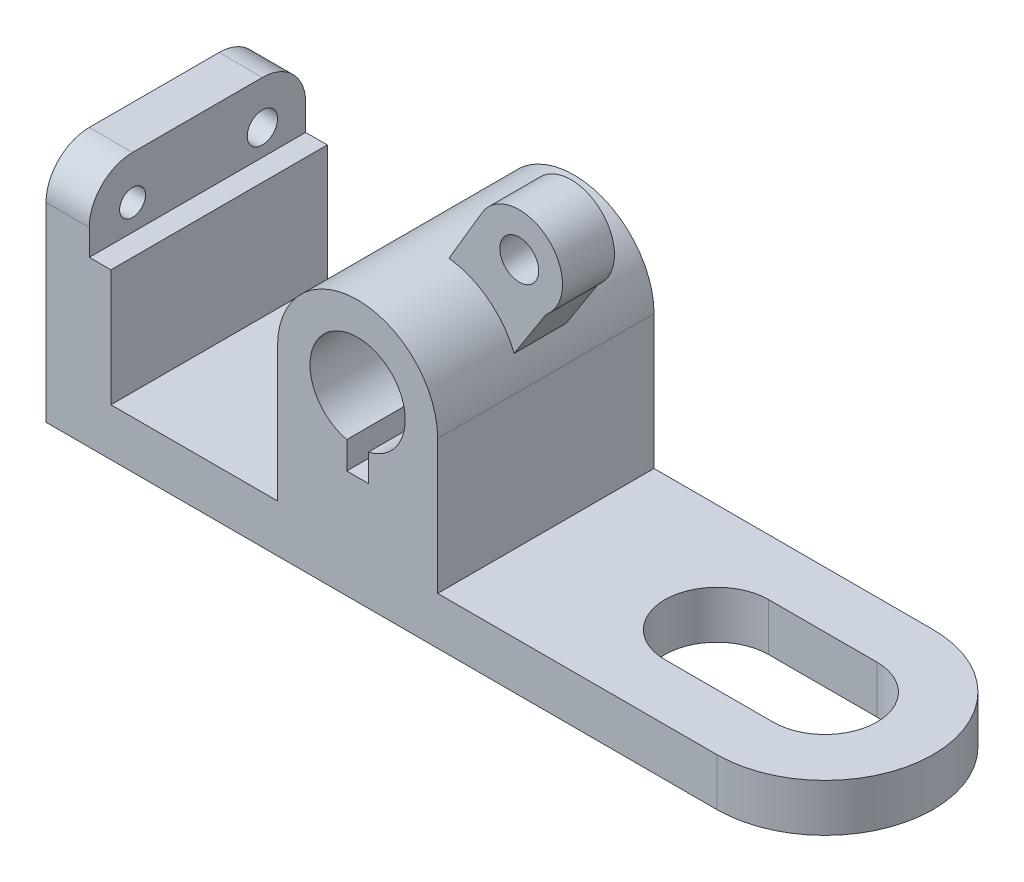
ISO-10303-21;
HEADER;
FILE_DESCRIPTION(('STEP AP214'),'2;1');
FILE_NAME('part.step','',(''),(''),'','','');
FILE_SCHEMA(('AUTOMOTIVE_DESIGN { 1 0 10303 214 1 1 1 1 }'));
ENDSEC;
DATA;
#1=APPLICATION_CONTEXT('core data for automotive mechanical design processes');
#2=APPLICATION_PROTOCOL_DEFINITION('international standard','automotive_design',2000,#1);
#3=PRODUCT_CONTEXT('',#1,'mechanical');
#4=PRODUCT('Part','Part','',(#3));
#5=PRODUCT_RELATED_PRODUCT_CATEGORY('part','',(#4));
#6=PRODUCT_DEFINITION_FORMATION('','',#4);
#7=PRODUCT_DEFINITION_CONTEXT('part definition',#1,'design');
#8=PRODUCT_DEFINITION('design','',#6,#7);
#9=PRODUCT_DEFINITION_SHAPE('','',#8);
#10=(LENGTH_UNIT() NAMED_UNIT(*) SI_UNIT(.MILLI.,.METRE.));
#11=(NAMED_UNIT(*) PLANE_ANGLE_UNIT() SI_UNIT($,.RADIAN.));
#12=(NAMED_UNIT(*) SI_UNIT($,.STERADIAN.) SOLID_ANGLE_UNIT());
#13=UNCERTAINTY_MEASURE_WITH_UNIT(LENGTH_MEASURE(1.E-05),#10,'distance_accuracy_value','');
#14=(GEOMETRIC_REPRESENTATION_CONTEXT(3) GLOBAL_UNCERTAINTY_ASSIGNED_CONTEXT((#13)) GLOBAL_UNIT_ASSIGNED_CONTEXT((#10,
#11,#12)) REPRESENTATION_CONTEXT('',''));
#15=CARTESIAN_POINT('',(0.,0.,0.));
#16=DIRECTION('',(0.,0.,1.));
#17=DIRECTION('',(1.,0.,0.));
#18=AXIS2_PLACEMENT_3D('',#15,#16,#17);
#19=CARTESIAN_POINT('',(-77.5,44.,-15.));
#20=DIRECTION('',(-1.,0.,0.));
#21=DIRECTION('',(0.,0.,1.));
#22=AXIS2_PLACEMENT_3D('',#19,#20,#21);
#23=CYLINDRICAL_SURFACE('',#22,10.);
#24=DIRECTION('',(1.,0.,0.));
#25=VECTOR('',#24,1.);
#26=CARTESIAN_POINT('',(-77.5,44.,-25.));
#27=LINE('',#26,#25);
#28=CARTESIAN_POINT('',(-77.5,44.,-25.));
#29=VERTEX_POINT('',#28);
#30=CARTESIAN_POINT('',(-67.5,44.,-25.));
#31=VERTEX_POINT('',#30);
#32=EDGE_CURVE('E419',#29,#31,#27,.T.);
#33=ORIENTED_EDGE('',*,*,#32,.F.);
#34=CARTESIAN_POINT('',(-77.5,44.,-15.));
#35=DIRECTION('',(1.,0.,0.));
#36=DIRECTION('',(0.,0.,-1.));
#37=AXIS2_PLACEMENT_3D('',#34,#35,#36);
#38=CIRCLE('',#37,10.);
#39=CARTESIAN_POINT('',(-77.5,54.,-15.));
#40=VERTEX_POINT('',#39);
#41=EDGE_CURVE('E11',#40,#29,#38,.F.);
#42=ORIENTED_EDGE('',*,*,#41,.F.);
#43=DIRECTION('',(1.,0.,0.));
#44=VECTOR('',#43,1.);
#45=CARTESIAN_POINT('',(-77.5,54.,-15.));
#46=LINE('',#45,#44);
#47=CARTESIAN_POINT('',(-67.5,54.,-15.));
#48=VERTEX_POINT('',#47);
#49=EDGE_CURVE('E47',#48,#40,#46,.F.);
#50=ORIENTED_EDGE('',*,*,#49,.F.);
#51=CARTESIAN_POINT('',(-67.5,44.,-15.));
#52=DIRECTION('',(1.,0.,0.));
#53=DIRECTION('',(0.,0.,-1.));
#54=AXIS2_PLACEMENT_3D('',#51,#52,#53);
#55=CIRCLE('',#54,10.);
#56=EDGE_CURVE('E421',#31,#48,#55,.T.);
#57=ORIENTED_EDGE('',*,*,#56,.F.);
#58=EDGE_LOOP('',(#33,#42,#50,#57));
#59=FACE_BOUND('',#58,.T.);
#60=ADVANCED_FACE('F41',(#59),#23,.T.);
#61=CARTESIAN_POINT('',(77.5,44.,15.));
#62=DIRECTION('',(1.,0.,0.));
#63=DIRECTION('',(0.,0.,-1.));
#64=AXIS2_PLACEMENT_3D('',#61,#62,#63);
#65=CYLINDRICAL_SURFACE('',#64,10.);
#66=DIRECTION('',(-1.,0.,0.));
#67=VECTOR('',#66,1.);
#68=CARTESIAN_POINT('',(77.5,44.,25.));
#69=LINE('',#68,#67);
#70=CARTESIAN_POINT('',(-67.5,44.,25.));
#71=VERTEX_POINT('',#70);
#72=CARTESIAN_POINT('',(-77.5,44.,25.));
#73=VERTEX_POINT('',#72);
#74=EDGE_CURVE('E413',#71,#73,#69,.T.);
#75=ORIENTED_EDGE('',*,*,#74,.F.);
#76=CARTESIAN_POINT('',(-67.5,44.,15.));
#77=DIRECTION('',(1.,0.,0.));
#78=DIRECTION('',(0.,0.,-1.));
#79=AXIS2_PLACEMENT_3D('',#76,#77,#78);
#80=CIRCLE('',#79,10.);
#81=CARTESIAN_POINT('',(-67.5,54.,15.));
#82=VERTEX_POINT('',#81);
#83=EDGE_CURVE('E240',#82,#71,#80,.T.);
#84=ORIENTED_EDGE('',*,*,#83,.F.);
#85=DIRECTION('',(-1.,0.,0.));
#86=VECTOR('',#85,1.);
#87=CARTESIAN_POINT('',(77.5,54.,15.));
#88=LINE('',#87,#86);
#89=CARTESIAN_POINT('',(-77.5,54.,15.));
#90=VERTEX_POINT('',#89);
#91=EDGE_CURVE('E412',#90,#82,#88,.F.);
#92=ORIENTED_EDGE('',*,*,#91,.F.);
#93=CARTESIAN_POINT('',(-77.5,44.,15.));
#94=DIRECTION('',(1.,0.,0.));
#95=DIRECTION('',(0.,0.,-1.));
#96=AXIS2_PLACEMENT_3D('',#93,#94,#95);
#97=CIRCLE('',#96,10.);
#98=EDGE_CURVE('E420',#73,#90,#97,.F.);
#99=ORIENTED_EDGE('',*,*,#98,.F.);
#100=EDGE_LOOP('',(#75,#84,#92,#99));
#101=FACE_BOUND('',#100,.T.);
#102=ADVANCED_FACE('F451',(#101),#65,.T.);
#103=CARTESIAN_POINT('',(77.5,11.,0.));
#104=DIRECTION('',(0.,1.,0.));
#105=DIRECTION('',(0.,0.,1.));
#106=AXIS2_PLACEMENT_3D('',#103,#104,#105);
#107=PLANE('',#106);
#108=DIRECTION('',(-1.,0.,0.));
#109=VECTOR('',#108,1.);
#110=CARTESIAN_POINT('',(-77.5,11.,-25.));
#111=LINE('',#110,#109);
#112=CARTESIAN_POINT('',(-24.,11.,-25.));
#113=VERTEX_POINT('',#112);
#114=CARTESIAN_POINT('',(-62.5,11.,-25.));
#115=VERTEX_POINT('',#114);
#116=EDGE_CURVE('E368',#113,#115,#111,.T.);
#117=ORIENTED_EDGE('',*,*,#116,.T.);
#118=DIRECTION('',(0.,0.,-1.));
#119=VECTOR('',#118,1.);
#120=CARTESIAN_POINT('',(-62.5,11.,25.));
#121=LINE('',#120,#119);
#122=CARTESIAN_POINT('',(-62.5,11.,25.));
#123=VERTEX_POINT('',#122);
#124=EDGE_CURVE('E225',#123,#115,#121,.T.);
#125=ORIENTED_EDGE('',*,*,#124,.F.);
#126=DIRECTION('',(1.,0.,0.));
#127=VECTOR('',#126,1.);
#128=CARTESIAN_POINT('',(77.5,11.,25.));
#129=LINE('',#128,#127);
#130=CARTESIAN_POINT('',(-24.,11.,25.));
#131=VERTEX_POINT('',#130);
#132=EDGE_CURVE('E367',#123,#131,#129,.T.);
#133=ORIENTED_EDGE('',*,*,#132,.T.);
#134=DIRECTION('',(0.,0.,1.));
#135=VECTOR('',#134,1.);
#136=CARTESIAN_POINT('',(-24.,11.,-25.));
#137=LINE('',#136,#135);
#138=EDGE_CURVE('E356',#113,#131,#137,.T.);
#139=ORIENTED_EDGE('',*,*,#138,.F.);
#140=EDGE_LOOP('',(#117,#125,#133,#139));
#141=FACE_BOUND('',#140,.T.);
#142=ADVANCED_FACE('F494',(#141),#107,.T.);
#143=CARTESIAN_POINT('',(77.5,11.,0.));
#144=DIRECTION('',(0.,1.,0.));
#145=DIRECTION('',(0.,0.,1.));
#146=AXIS2_PLACEMENT_3D('',#143,#144,#145);
#147=CIRCLE('',#146,12.);
#148=CARTESIAN_POINT('',(77.5000000000001,11.,12.));
#149=VERTEX_POINT('',#148);
#150=CARTESIAN_POINT('',(77.5,11.,-12.));
#151=VERTEX_POINT('',#150);
#152=EDGE_CURVE('E259',#149,#151,#147,.T.);
#153=ORIENTED_EDGE('',*,*,#152,.F.);
#154=DIRECTION('',(1.,0.,0.));
#155=VECTOR('',#154,1.);
#156=CARTESIAN_POINT('',(52.5,11.,12.));
#157=LINE('',#156,#155);
#158=CARTESIAN_POINT('',(52.5,11.,12.));
#159=VERTEX_POINT('',#158);
#160=EDGE_CURVE('E265',#159,#149,#157,.T.);
#161=ORIENTED_EDGE('',*,*,#160,.F.);
#162=CARTESIAN_POINT('',(52.5,11.,0.));
#163=DIRECTION('',(0.,1.,0.));
#164=DIRECTION('',(0.,0.,1.));
#165=AXIS2_PLACEMENT_3D('',#162,#163,#164);
#166=CIRCLE('',#165,12.);
#167=CARTESIAN_POINT('',(52.5,11.,-12.));
#168=VERTEX_POINT('',#167);
#169=EDGE_CURVE('E263',#168,#159,#166,.T.);
#170=ORIENTED_EDGE('',*,*,#169,.F.);
#171=DIRECTION('',(-1.,0.,0.));
#172=VECTOR('',#171,1.);
#173=CARTESIAN_POINT('',(52.5,11.,-12.));
#174=LINE('',#173,#172);
#175=EDGE_CURVE('E260',#151,#168,#174,.T.);
#176=ORIENTED_EDGE('',*,*,#175,.F.);
#177=EDGE_LOOP('',(#153,#161,#170,#176));
#178=FACE_BOUND('',#177,.T.);
#179=CARTESIAN_POINT('',(77.5,11.,-25.));
#180=VERTEX_POINT('',#179);
#181=CARTESIAN_POINT('',(13.,11.,-25.));
#182=VERTEX_POINT('',#181);
#183=EDGE_CURVE('E364',#180,#182,#111,.T.);
#184=ORIENTED_EDGE('',*,*,#183,.T.);
#185=DIRECTION('',(0.,0.,1.));
#186=VECTOR('',#185,1.);
#187=CARTESIAN_POINT('',(13.,11.,-25.));
#188=LINE('',#187,#186);
#189=CARTESIAN_POINT('',(13.,11.,25.));
#190=VERTEX_POINT('',#189);
#191=EDGE_CURVE('E352',#182,#190,#188,.T.);
#192=ORIENTED_EDGE('',*,*,#191,.T.);
#193=CARTESIAN_POINT('',(77.5,11.,25.));
#194=VERTEX_POINT('',#193);
#195=EDGE_CURVE('E370',#190,#194,#129,.T.);
#196=ORIENTED_EDGE('',*,*,#195,.T.);
#197=CARTESIAN_POINT('',(77.5,11.,0.));
#198=DIRECTION('',(0.,1.,0.));
#199=DIRECTION('',(0.,0.,1.));
#200=AXIS2_PLACEMENT_3D('',#197,#198,#199);
#201=CIRCLE('',#200,25.);
#202=EDGE_CURVE('E371',#194,#180,#201,.T.);
#203=ORIENTED_EDGE('',*,*,#202,.T.);
#204=EDGE_LOOP('',(#184,#192,#196,#203));
#205=FACE_BOUND('',#204,.T.);
#206=ADVANCED_FACE('F466',(#178,#205),#107,.T.);
#207=CARTESIAN_POINT('',(-77.5,11.,-25.));
#208=DIRECTION('',(0.,0.,1.));
#209=DIRECTION('',(1.,0.,0.));
#210=AXIS2_PLACEMENT_3D('',#207,#208,#209);
#211=PLANE('',#210);
#212=DIRECTION('',(-1.,0.,0.));
#213=VECTOR('',#212,1.);
#214=CARTESIAN_POINT('',(-5.5,25.,-25.));
#215=LINE('',#214,#213);
#216=CARTESIAN_POINT('',(-3.,25.,-25.));
#217=VERTEX_POINT('',#216);
#218=CARTESIAN_POINT('',(-8.,25.,-25.));
#219=VERTEX_POINT('',#218);
#220=EDGE_CURVE('E319',#217,#219,#215,.T.);
#221=ORIENTED_EDGE('',*,*,#220,.F.);
#222=DIRECTION('',(0.,1.,0.));
#223=VECTOR('',#222,1.);
#224=CARTESIAN_POINT('',(-3.,25.,-25.));
#225=LINE('',#224,#223);
#226=CARTESIAN_POINT('',(-3.,31.2878573571857,-25.));
#227=VERTEX_POINT('',#226);
#228=EDGE_CURVE('E308',#217,#227,#225,.T.);
#229=ORIENTED_EDGE('',*,*,#228,.T.);
#230=CARTESIAN_POINT('',(-5.50000000000001,42.,-25.));
#231=DIRECTION('',(0.,0.,1.));
#232=DIRECTION('',(1.,0.,0.));
#233=AXIS2_PLACEMENT_3D('',#230,#231,#232);
#234=CIRCLE('',#233,11.);
#235=CARTESIAN_POINT('',(-8.,31.2878573571857,-25.));
#236=VERTEX_POINT('',#235);
#237=EDGE_CURVE('E311',#227,#236,#234,.T.);
#238=ORIENTED_EDGE('',*,*,#237,.T.);
#239=DIRECTION('',(0.,1.,0.));
#240=VECTOR('',#239,1.);
#241=CARTESIAN_POINT('',(-8.,25.,-25.));
#242=LINE('',#241,#240);
#243=EDGE_CURVE('E314',#219,#236,#242,.T.);
#244=ORIENTED_EDGE('',*,*,#243,.F.);
#245=EDGE_LOOP('',(#221,#229,#238,#244));
#246=FACE_BOUND('',#245,.T.);
#247=DIRECTION('',(0.,-1.,0.));
#248=VECTOR('',#247,1.);
#249=CARTESIAN_POINT('',(-77.5,11.,-25.));
#250=LINE('',#249,#248);
#251=CARTESIAN_POINT('',(-77.5,0.,-25.));
#252=VERTEX_POINT('',#251);
#253=EDGE_CURVE('E387',#29,#252,#250,.T.);
#254=ORIENTED_EDGE('',*,*,#253,.F.);
#255=ORIENTED_EDGE('',*,*,#32,.T.);
#256=DIRECTION('',(0.,1.,0.));
#257=VECTOR('',#256,1.);
#258=CARTESIAN_POINT('',(-67.5,38.,-25.));
#259=LINE('',#258,#257);
#260=CARTESIAN_POINT('',(-67.5,38.,-25.));
#261=VERTEX_POINT('',#260);
#262=EDGE_CURVE('E231',#261,#31,#259,.T.);
#263=ORIENTED_EDGE('',*,*,#262,.F.);
#264=DIRECTION('',(-1.,0.,0.));
#265=VECTOR('',#264,1.);
#266=CARTESIAN_POINT('',(-62.5,38.,-25.));
#267=LINE('',#266,#265);
#268=CARTESIAN_POINT('',(-62.5,38.,-25.));
#269=VERTEX_POINT('',#268);
#270=EDGE_CURVE('E226',#269,#261,#267,.T.);
#271=ORIENTED_EDGE('',*,*,#270,.F.);
#272=DIRECTION('',(0.,-1.,0.));
#273=VECTOR('',#272,1.);
#274=CARTESIAN_POINT('',(-62.5,38.,-25.));
#275=LINE('',#274,#273);
#276=EDGE_CURVE('E249',#269,#115,#275,.T.);
#277=ORIENTED_EDGE('',*,*,#276,.T.);
#278=ORIENTED_EDGE('',*,*,#116,.F.);
#279=DIRECTION('',(0.,-1.,0.));
#280=VECTOR('',#279,1.);
#281=CARTESIAN_POINT('',(-24.,0.,-25.));
#282=LINE('',#281,#280);
#283=CARTESIAN_POINT('',(-24.,42.,-25.));
#284=VERTEX_POINT('',#283);
#285=EDGE_CURVE('E342',#284,#113,#282,.T.);
#286=ORIENTED_EDGE('',*,*,#285,.F.);
#287=CARTESIAN_POINT('',(-5.50000000000001,42.,-25.));
#288=DIRECTION('',(0.,0.,1.));
#289=DIRECTION('',(1.,0.,0.));
#290=AXIS2_PLACEMENT_3D('',#287,#288,#289);
#291=CIRCLE('',#290,18.5);
#292=CARTESIAN_POINT('',(13.,42.,-25.));
#293=VERTEX_POINT('',#292);
#294=EDGE_CURVE('E344',#293,#284,#291,.T.);
#295=ORIENTED_EDGE('',*,*,#294,.F.);
#296=DIRECTION('',(0.,-1.,0.));
#297=VECTOR('',#296,1.);
#298=CARTESIAN_POINT('',(13.,0.,-25.));
#299=LINE('',#298,#297);
#300=EDGE_CURVE('E339',#293,#182,#299,.T.);
#301=ORIENTED_EDGE('',*,*,#300,.T.);
#302=ORIENTED_EDGE('',*,*,#183,.F.);
#303=DIRECTION('',(0.,-1.,0.));
#304=VECTOR('',#303,1.);
#305=CARTESIAN_POINT('',(77.5,11.,-25.));
#306=LINE('',#305,#304);
#307=CARTESIAN_POINT('',(77.5,0.,-25.));
#308=VERTEX_POINT('',#307);
#309=EDGE_CURVE('E373',#180,#308,#306,.T.);
#310=ORIENTED_EDGE('',*,*,#309,.T.);
#311=DIRECTION('',(-1.,0.,0.));
#312=VECTOR('',#311,1.);
#313=CARTESIAN_POINT('',(-77.5,0.,-25.));
#314=LINE('',#313,#312);
#315=EDGE_CURVE('E357',#308,#252,#314,.T.);
#316=ORIENTED_EDGE('',*,*,#315,.T.);
#317=EDGE_LOOP('',(#254,#255,#263,#271,#277,#278,#286,#295,#301,#302,#310,#316));
#318=FACE_BOUND('',#317,.T.);
#319=ADVANCED_FACE('F445',(#246,#318),#211,.F.);
#320=CARTESIAN_POINT('',(-77.5,11.,-25.));
#321=DIRECTION('',(1.,0.,0.));
#322=DIRECTION('',(0.,0.,-1.));
#323=AXIS2_PLACEMENT_3D('',#320,#321,#322);
#324=PLANE('',#323);
#325=CARTESIAN_POINT('',(-77.5,44.,-15.));
#326=DIRECTION('',(-1.,0.,0.));
#327=DIRECTION('',(0.,0.,1.));
#328=AXIS2_PLACEMENT_3D('',#325,#326,#327);
#329=CIRCLE('',#328,3.5);
#330=CARTESIAN_POINT('',(-77.5,44.,-11.5));
#331=VERTEX_POINT('',#330);
#332=EDGE_CURVE('E428',#331,#331,#329,.T.);
#333=ORIENTED_EDGE('',*,*,#332,.F.);
#334=EDGE_LOOP('',(#333));
#335=FACE_BOUND('',#334,.T.);
#336=CARTESIAN_POINT('',(-77.5,44.,15.));
#337=DIRECTION('',(-1.,0.,0.));
#338=DIRECTION('',(0.,0.,1.));
#339=AXIS2_PLACEMENT_3D('',#336,#337,#338);
#340=CIRCLE('',#339,3.);
#341=CARTESIAN_POINT('',(-77.5,44.,18.));
#342=VERTEX_POINT('',#341);
#343=EDGE_CURVE('E427',#342,#342,#340,.T.);
#344=ORIENTED_EDGE('',*,*,#343,.F.);
#345=EDGE_LOOP('',(#344));
#346=FACE_BOUND('',#345,.T.);
#347=DIRECTION('',(0.,0.,1.));
#348=VECTOR('',#347,1.);
#349=CARTESIAN_POINT('',(-77.5,54.,-25.));
#350=LINE('',#349,#348);
#351=EDGE_CURVE('E244',#40,#90,#350,.T.);
#352=ORIENTED_EDGE('',*,*,#351,.F.);
#353=ORIENTED_EDGE('',*,*,#41,.T.);
#354=ORIENTED_EDGE('',*,*,#253,.T.);
#355=DIRECTION('',(0.,0.,1.));
#356=VECTOR('',#355,1.);
#357=CARTESIAN_POINT('',(-77.5,0.,-25.));
#358=LINE('',#357,#356);
#359=CARTESIAN_POINT('',(-77.5,0.,25.));
#360=VERTEX_POINT('',#359);
#361=EDGE_CURVE('E376',#252,#360,#358,.T.);
#362=ORIENTED_EDGE('',*,*,#361,.T.);
#363=DIRECTION('',(0.,-1.,0.));
#364=VECTOR('',#363,1.);
#365=CARTESIAN_POINT('',(-77.5,11.,25.));
#366=LINE('',#365,#364);
#367=EDGE_CURVE('E390',#73,#360,#366,.T.);
#368=ORIENTED_EDGE('',*,*,#367,.F.);
#369=ORIENTED_EDGE('',*,*,#98,.T.);
#370=EDGE_LOOP('',(#352,#353,#354,#362,#368,#369));
#371=FACE_BOUND('',#370,.T.);
#372=ADVANCED_FACE('F437',(#335,#346,#371),#324,.F.);
#373=CARTESIAN_POINT('',(77.5,11.,25.));
#374=DIRECTION('',(0.,0.,-1.));
#375=DIRECTION('',(-1.,0.,0.));
#376=AXIS2_PLACEMENT_3D('',#373,#374,#375);
#377=PLANE('',#376);
#378=CARTESIAN_POINT('',(-5.50000000000001,42.,25.));
#379=DIRECTION('',(0.,0.,1.));
#380=DIRECTION('',(1.,0.,0.));
#381=AXIS2_PLACEMENT_3D('',#378,#379,#380);
#382=CIRCLE('',#381,11.);
#383=CARTESIAN_POINT('',(-3.,31.2878573571857,25.));
#384=VERTEX_POINT('',#383);
#385=CARTESIAN_POINT('',(-8.,31.2878573571857,25.));
#386=VERTEX_POINT('',#385);
#387=EDGE_CURVE('E321',#384,#386,#382,.T.);
#388=ORIENTED_EDGE('',*,*,#387,.F.);
#389=DIRECTION('',(0.,1.,0.));
#390=VECTOR('',#389,1.);
#391=CARTESIAN_POINT('',(-3.,25.,25.));
#392=LINE('',#391,#390);
#393=CARTESIAN_POINT('',(-3.,25.,25.));
#394=VERTEX_POINT('',#393);
#395=EDGE_CURVE('E310',#394,#384,#392,.T.);
#396=ORIENTED_EDGE('',*,*,#395,.F.);
#397=DIRECTION('',(1.,0.,0.));
#398=VECTOR('',#397,1.);
#399=CARTESIAN_POINT('',(-5.5,25.,25.));
#400=LINE('',#399,#398);
#401=CARTESIAN_POINT('',(-8.,25.,25.));
#402=VERTEX_POINT('',#401);
#403=EDGE_CURVE('E315',#402,#394,#400,.T.);
#404=ORIENTED_EDGE('',*,*,#403,.F.);
#405=DIRECTION('',(0.,1.,0.));
#406=VECTOR('',#405,1.);
#407=CARTESIAN_POINT('',(-8.,25.,25.));
#408=LINE('',#407,#406);
#409=EDGE_CURVE('E322',#402,#386,#408,.T.);
#410=ORIENTED_EDGE('',*,*,#409,.T.);
#411=EDGE_LOOP('',(#388,#396,#404,#410));
#412=FACE_BOUND('',#411,.T.);
#413=DIRECTION('',(0.,1.,0.));
#414=VECTOR('',#413,1.);
#415=CARTESIAN_POINT('',(-67.5,38.,25.));
#416=LINE('',#415,#414);
#417=CARTESIAN_POINT('',(-67.5,38.,25.));
#418=VERTEX_POINT('',#417);
#419=EDGE_CURVE('E212',#418,#71,#416,.T.);
#420=ORIENTED_EDGE('',*,*,#419,.T.);
#421=ORIENTED_EDGE('',*,*,#74,.T.);
#422=ORIENTED_EDGE('',*,*,#367,.T.);
#423=DIRECTION('',(1.,0.,0.));
#424=VECTOR('',#423,1.);
#425=CARTESIAN_POINT('',(77.5,0.,25.));
#426=LINE('',#425,#424);
#427=CARTESIAN_POINT('',(77.5,0.,25.));
#428=VERTEX_POINT('',#427);
#429=EDGE_CURVE('E378',#360,#428,#426,.T.);
#430=ORIENTED_EDGE('',*,*,#429,.T.);
#431=DIRECTION('',(0.,-1.,0.));
#432=VECTOR('',#431,1.);
#433=CARTESIAN_POINT('',(77.5,11.,25.));
#434=LINE('',#433,#432);
#435=EDGE_CURVE('E383',#194,#428,#434,.T.);
#436=ORIENTED_EDGE('',*,*,#435,.F.);
#437=ORIENTED_EDGE('',*,*,#195,.F.);
#438=DIRECTION('',(0.,-1.,0.));
#439=VECTOR('',#438,1.);
#440=CARTESIAN_POINT('',(13.,0.,25.));
#441=LINE('',#440,#439);
#442=CARTESIAN_POINT('',(13.,42.,25.));
#443=VERTEX_POINT('',#442);
#444=EDGE_CURVE('E335',#443,#190,#441,.T.);
#445=ORIENTED_EDGE('',*,*,#444,.F.);
#446=CARTESIAN_POINT('',(-5.50000000000001,42.,25.));
#447=DIRECTION('',(0.,0.,1.));
#448=DIRECTION('',(1.,0.,0.));
#449=AXIS2_PLACEMENT_3D('',#446,#447,#448);
#450=CIRCLE('',#449,18.5);
#451=CARTESIAN_POINT('',(-24.,42.,25.));
#452=VERTEX_POINT('',#451);
#453=EDGE_CURVE('E350',#443,#452,#450,.T.);
#454=ORIENTED_EDGE('',*,*,#453,.T.);
#455=DIRECTION('',(0.,-1.,0.));
#456=VECTOR('',#455,1.);
#457=CARTESIAN_POINT('',(-24.,0.,25.));
#458=LINE('',#457,#456);
#459=EDGE_CURVE('E341',#452,#131,#458,.T.);
#460=ORIENTED_EDGE('',*,*,#459,.T.);
#461=ORIENTED_EDGE('',*,*,#132,.F.);
#462=DIRECTION('',(0.,-1.,0.));
#463=VECTOR('',#462,1.);
#464=CARTESIAN_POINT('',(-62.5,38.,25.));
#465=LINE('',#464,#463);
#466=CARTESIAN_POINT('',(-62.5,38.,25.));
#467=VERTEX_POINT('',#466);
#468=EDGE_CURVE('E217',#467,#123,#465,.T.);
#469=ORIENTED_EDGE('',*,*,#468,.F.);
#470=DIRECTION('',(1.,0.,0.));
#471=VECTOR('',#470,1.);
#472=CARTESIAN_POINT('',(-77.5,38.,25.));
#473=LINE('',#472,#471);
#474=EDGE_CURVE('E208',#418,#467,#473,.T.);
#475=ORIENTED_EDGE('',*,*,#474,.F.);
#476=EDGE_LOOP('',(#420,#421,#422,#430,#436,#437,#445,#454,#460,#461,#469,#475));
#477=FACE_BOUND('',#476,.T.);
#478=ADVANCED_FACE('F211',(#412,#477),#377,.F.);
#479=CARTESIAN_POINT('',(77.5,11.,0.));
#480=DIRECTION('',(0.,-1.,0.));
#481=DIRECTION('',(0.,0.,-1.));
#482=AXIS2_PLACEMENT_3D('',#479,#480,#481);
#483=CYLINDRICAL_SURFACE('',#482,25.);
#484=CARTESIAN_POINT('',(77.5,0.,0.));
#485=DIRECTION('',(0.,1.,0.));
#486=DIRECTION('',(0.,0.,1.));
#487=AXIS2_PLACEMENT_3D('',#484,#485,#486);
#488=CIRCLE('',#487,25.);
#489=EDGE_CURVE('E382',#428,#308,#488,.T.);
#490=ORIENTED_EDGE('',*,*,#489,.T.);
#491=ORIENTED_EDGE('',*,*,#309,.F.);
#492=ORIENTED_EDGE('',*,*,#202,.F.);
#493=ORIENTED_EDGE('',*,*,#435,.T.);
#494=EDGE_LOOP('',(#490,#491,#492,#493));
#495=FACE_BOUND('',#494,.T.);
#496=ADVANCED_FACE('F462',(#495),#483,.T.);
#497=CARTESIAN_POINT('',(77.5,0.,0.));
#498=DIRECTION('',(0.,1.,0.));
#499=DIRECTION('',(0.,0.,1.));
#500=AXIS2_PLACEMENT_3D('',#497,#498,#499);
#501=PLANE('',#500);
#502=DIRECTION('',(1.,0.,0.));
#503=VECTOR('',#502,1.);
#504=CARTESIAN_POINT('',(77.5,0.,12.));
#505=LINE('',#504,#503);
#506=CARTESIAN_POINT('',(52.5,0.,12.));
#507=VERTEX_POINT('',#506);
#508=CARTESIAN_POINT('',(77.5000000000001,0.,12.));
#509=VERTEX_POINT('',#508);
#510=EDGE_CURVE('E403',#507,#509,#505,.T.);
#511=ORIENTED_EDGE('',*,*,#510,.T.);
#512=CARTESIAN_POINT('',(77.5,0.,0.));
#513=DIRECTION('',(0.,1.,0.));
#514=DIRECTION('',(0.,0.,1.));
#515=AXIS2_PLACEMENT_3D('',#512,#513,#514);
#516=CIRCLE('',#515,12.);
#517=CARTESIAN_POINT('',(77.5,0.,-12.));
#518=VERTEX_POINT('',#517);
#519=EDGE_CURVE('E410',#509,#518,#516,.T.);
#520=ORIENTED_EDGE('',*,*,#519,.T.);
#521=DIRECTION('',(-1.,0.,0.));
#522=VECTOR('',#521,1.);
#523=CARTESIAN_POINT('',(77.5,0.,-12.));
#524=LINE('',#523,#522);
#525=CARTESIAN_POINT('',(52.5,0.,-12.));
#526=VERTEX_POINT('',#525);
#527=EDGE_CURVE('E400',#518,#526,#524,.T.);
#528=ORIENTED_EDGE('',*,*,#527,.T.);
#529=CARTESIAN_POINT('',(52.5,0.,0.));
#530=DIRECTION('',(0.,1.,0.));
#531=DIRECTION('',(0.,0.,1.));
#532=AXIS2_PLACEMENT_3D('',#529,#530,#531);
#533=CIRCLE('',#532,12.);
#534=EDGE_CURVE('E405',#526,#507,#533,.T.);
#535=ORIENTED_EDGE('',*,*,#534,.T.);
#536=EDGE_LOOP('',(#511,#520,#528,#535));
#537=FACE_BOUND('',#536,.T.);
#538=ORIENTED_EDGE('',*,*,#315,.F.);
#539=ORIENTED_EDGE('',*,*,#489,.F.);
#540=ORIENTED_EDGE('',*,*,#429,.F.);
#541=ORIENTED_EDGE('',*,*,#361,.F.);
#542=EDGE_LOOP('',(#538,#539,#540,#541));
#543=FACE_BOUND('',#542,.T.);
#544=ADVANCED_FACE('F460',(#537,#543),#501,.F.);
#545=CARTESIAN_POINT('',(13.,0.,-25.));
#546=DIRECTION('',(-1.,0.,0.));
#547=DIRECTION('',(0.,-1.,0.));
#548=AXIS2_PLACEMENT_3D('',#545,#546,#547);
#549=PLANE('',#548);
#550=ORIENTED_EDGE('',*,*,#444,.T.);
#551=ORIENTED_EDGE('',*,*,#191,.F.);
#552=ORIENTED_EDGE('',*,*,#300,.F.);
#553=DIRECTION('',(0.,0.,1.));
#554=VECTOR('',#553,1.);
#555=CARTESIAN_POINT('',(13.,42.,-25.));
#556=LINE('',#555,#554);
#557=EDGE_CURVE('E349',#293,#443,#556,.T.);
#558=ORIENTED_EDGE('',*,*,#557,.T.);
#559=EDGE_LOOP('',(#550,#551,#552,#558));
#560=FACE_BOUND('',#559,.T.);
#561=ADVANCED_FACE('F507',(#560),#549,.F.);
#562=CARTESIAN_POINT('',(-24.,0.,-25.));
#563=DIRECTION('',(-1.,0.,0.));
#564=DIRECTION('',(0.,-1.,0.));
#565=AXIS2_PLACEMENT_3D('',#562,#563,#564);
#566=PLANE('',#565);
#567=ORIENTED_EDGE('',*,*,#459,.F.);
#568=DIRECTION('',(0.,0.,1.));
#569=VECTOR('',#568,1.);
#570=CARTESIAN_POINT('',(-24.,42.,-25.));
#571=LINE('',#570,#569);
#572=EDGE_CURVE('E363',#284,#452,#571,.T.);
#573=ORIENTED_EDGE('',*,*,#572,.F.);
#574=ORIENTED_EDGE('',*,*,#285,.T.);
#575=ORIENTED_EDGE('',*,*,#138,.T.);
#576=EDGE_LOOP('',(#567,#573,#574,#575));
#577=FACE_BOUND('',#576,.T.);
#578=ADVANCED_FACE('F476',(#577),#566,.T.);
#579=CARTESIAN_POINT('',(-5.50000000000001,42.,-25.));
#580=DIRECTION('',(0.,0.,1.));
#581=DIRECTION('',(1.,0.,0.));
#582=AXIS2_PLACEMENT_3D('',#579,#580,#581);
#583=CYLINDRICAL_SURFACE('',#582,18.5);
#584=CARTESIAN_POINT('',(-5.50000000000001,42.,6.));
#585=DIRECTION('',(0.,0.,1.));
#586=DIRECTION('',(1.,0.,0.));
#587=AXIS2_PLACEMENT_3D('',#584,#585,#586);
#588=CIRCLE('',#587,18.5);
#589=CARTESIAN_POINT('',(-3.37690232598644,60.3777707099256,6.));
#590=VERTEX_POINT('',#589);
#591=CARTESIAN_POINT('',(11.6741300156713,48.8774456162748,6.));
#592=VERTEX_POINT('',#591);
#593=EDGE_CURVE('E391',#590,#592,#588,.F.);
#594=ORIENTED_EDGE('',*,*,#593,.F.);
#595=DIRECTION('',(0.,0.,-1.));
#596=VECTOR('',#595,1.);
#597=CARTESIAN_POINT('',(-3.37690232598644,60.3777707099256,6.));
#598=LINE('',#597,#596);
#599=CARTESIAN_POINT('',(-3.37690232598644,60.3777707099256,-6.));
#600=VERTEX_POINT('',#599);
#601=EDGE_CURVE('E301',#590,#600,#598,.T.);
#602=ORIENTED_EDGE('',*,*,#601,.T.);
#603=CARTESIAN_POINT('',(-5.50000000000001,42.,-6.));
#604=DIRECTION('',(0.,0.,1.));
#605=DIRECTION('',(1.,0.,0.));
#606=AXIS2_PLACEMENT_3D('',#603,#604,#605);
#607=CIRCLE('',#606,18.5);
#608=CARTESIAN_POINT('',(11.6741300156713,48.8774456162748,-6.));
#609=VERTEX_POINT('',#608);
#610=EDGE_CURVE('E394',#600,#609,#607,.F.);
#611=ORIENTED_EDGE('',*,*,#610,.T.);
#612=DIRECTION('',(0.,0.,-1.));
#613=VECTOR('',#612,1.);
#614=CARTESIAN_POINT('',(11.6741300156713,48.8774456162748,6.));
#615=LINE('',#614,#613);
#616=EDGE_CURVE('E296',#592,#609,#615,.T.);
#617=ORIENTED_EDGE('',*,*,#616,.F.);
#618=EDGE_LOOP('',(#594,#602,#611,#617));
#619=FACE_BOUND('',#618,.T.);
#620=ORIENTED_EDGE('',*,*,#453,.F.);
#621=ORIENTED_EDGE('',*,*,#557,.F.);
#622=ORIENTED_EDGE('',*,*,#294,.T.);
#623=ORIENTED_EDGE('',*,*,#572,.T.);
#624=EDGE_LOOP('',(#620,#621,#622,#623));
#625=FACE_BOUND('',#624,.T.);
#626=ADVANCED_FACE('F473',(#619,#625),#583,.T.);
#627=CARTESIAN_POINT('',(-3.,25.,-25.));
#628=DIRECTION('',(1.,0.,0.));
#629=DIRECTION('',(0.,0.,-1.));
#630=AXIS2_PLACEMENT_3D('',#627,#628,#629);
#631=PLANE('',#630);
#632=ORIENTED_EDGE('',*,*,#395,.T.);
#633=DIRECTION('',(0.,0.,1.));
#634=VECTOR('',#633,1.);
#635=CARTESIAN_POINT('',(-3.,31.2878573571857,-25.));
#636=LINE('',#635,#634);
#637=EDGE_CURVE('E318',#227,#384,#636,.T.);
#638=ORIENTED_EDGE('',*,*,#637,.F.);
#639=ORIENTED_EDGE('',*,*,#228,.F.);
#640=DIRECTION('',(0.,0.,1.));
#641=VECTOR('',#640,1.);
#642=CARTESIAN_POINT('',(-3.,25.,-25.));
#643=LINE('',#642,#641);
#644=EDGE_CURVE('E326',#217,#394,#643,.T.);
#645=ORIENTED_EDGE('',*,*,#644,.T.);
#646=EDGE_LOOP('',(#632,#638,#639,#645));
#647=FACE_BOUND('',#646,.T.);
#648=ADVANCED_FACE('F513',(#647),#631,.F.);
#649=CARTESIAN_POINT('',(-5.5,25.,-25.));
#650=DIRECTION('',(0.,-1.,0.));
#651=DIRECTION('',(0.,0.,-1.));
#652=AXIS2_PLACEMENT_3D('',#649,#650,#651);
#653=PLANE('',#652);
#654=ORIENTED_EDGE('',*,*,#403,.T.);
#655=ORIENTED_EDGE('',*,*,#644,.F.);
#656=ORIENTED_EDGE('',*,*,#220,.T.);
#657=DIRECTION('',(0.,0.,1.));
#658=VECTOR('',#657,1.);
#659=CARTESIAN_POINT('',(-8.,25.,-25.));
#660=LINE('',#659,#658);
#661=EDGE_CURVE('E333',#219,#402,#660,.T.);
#662=ORIENTED_EDGE('',*,*,#661,.T.);
#663=EDGE_LOOP('',(#654,#655,#656,#662));
#664=FACE_BOUND('',#663,.T.);
#665=ADVANCED_FACE('F523',(#664),#653,.F.);
#666=CARTESIAN_POINT('',(-8.,25.,-25.));
#667=DIRECTION('',(1.,0.,0.));
#668=DIRECTION('',(0.,0.,-1.));
#669=AXIS2_PLACEMENT_3D('',#666,#667,#668);
#670=PLANE('',#669);
#671=ORIENTED_EDGE('',*,*,#409,.F.);
#672=ORIENTED_EDGE('',*,*,#661,.F.);
#673=ORIENTED_EDGE('',*,*,#243,.T.);
#674=DIRECTION('',(0.,0.,1.));
#675=VECTOR('',#674,1.);
#676=CARTESIAN_POINT('',(-8.,31.2878573571857,-25.));
#677=LINE('',#676,#675);
#678=EDGE_CURVE('E334',#236,#386,#677,.T.);
#679=ORIENTED_EDGE('',*,*,#678,.T.);
#680=EDGE_LOOP('',(#671,#672,#673,#679));
#681=FACE_BOUND('',#680,.T.);
#682=ADVANCED_FACE('F530',(#681),#670,.T.);
#683=CARTESIAN_POINT('',(-5.50000000000001,42.,-25.));
#684=DIRECTION('',(0.,0.,1.));
#685=DIRECTION('',(1.,0.,0.));
#686=AXIS2_PLACEMENT_3D('',#683,#684,#685);
#687=CYLINDRICAL_SURFACE('',#686,11.);
#688=ORIENTED_EDGE('',*,*,#387,.T.);
#689=ORIENTED_EDGE('',*,*,#678,.F.);
#690=ORIENTED_EDGE('',*,*,#237,.F.);
#691=ORIENTED_EDGE('',*,*,#637,.T.);
#692=EDGE_LOOP('',(#688,#689,#690,#691));
#693=FACE_BOUND('',#692,.T.);
#694=ADVANCED_FACE('F522',(#693),#687,.F.);
#695=CARTESIAN_POINT('',(12.8544459632334,68.2128654172478,6.));
#696=DIRECTION('',(0.,0.,-1.));
#697=DIRECTION('',(-1.,0.,0.));
#698=AXIS2_PLACEMENT_3D('',#695,#696,#697);
#699=CYLINDRICAL_SURFACE('',#698,9.99999999999999);
#700=CARTESIAN_POINT('',(12.8544459632334,68.2128654172478,-6.));
#701=DIRECTION('',(0.,0.,1.));
#702=DIRECTION('',(1.,0.,0.));
#703=AXIS2_PLACEMENT_3D('',#700,#701,#702);
#704=CIRCLE('',#703,9.99999999999999);
#705=CARTESIAN_POINT('',(19.0698001090793,60.3790047571572,-6.));
#706=VERTEX_POINT('',#705);
#707=CARTESIAN_POINT('',(4.24113224859956,73.2933011124712,-6.));
#708=VERTEX_POINT('',#707);
#709=EDGE_CURVE('E287',#706,#708,#704,.T.);
#710=ORIENTED_EDGE('',*,*,#709,.T.);
#711=DIRECTION('',(0.,0.,-1.));
#712=VECTOR('',#711,1.);
#713=CARTESIAN_POINT('',(4.24113224859956,73.2933011124712,6.));
#714=LINE('',#713,#712);
#715=CARTESIAN_POINT('',(4.24113224859956,73.2933011124712,6.));
#716=VERTEX_POINT('',#715);
#717=EDGE_CURVE('E302',#716,#708,#714,.T.);
#718=ORIENTED_EDGE('',*,*,#717,.F.);
#719=CARTESIAN_POINT('',(12.8544459632334,68.2128654172478,6.));
#720=DIRECTION('',(0.,0.,1.));
#721=DIRECTION('',(1.,0.,0.));
#722=AXIS2_PLACEMENT_3D('',#719,#720,#721);
#723=CIRCLE('',#722,9.99999999999999);
#724=CARTESIAN_POINT('',(19.0698001090793,60.3790047571572,6.));
#725=VERTEX_POINT('',#724);
#726=EDGE_CURVE('E277',#725,#716,#723,.T.);
#727=ORIENTED_EDGE('',*,*,#726,.F.);
#728=DIRECTION('',(0.,0.,-1.));
#729=VECTOR('',#728,1.);
#730=CARTESIAN_POINT('',(19.0698001090793,60.3790047571572,6.));
#731=LINE('',#730,#729);
#732=EDGE_CURVE('E288',#725,#706,#731,.T.);
#733=ORIENTED_EDGE('',*,*,#732,.T.);
#734=EDGE_LOOP('',(#710,#718,#727,#733));
#735=FACE_BOUND('',#734,.T.);
#736=ADVANCED_FACE('F526',(#735),#699,.T.);
#737=CARTESIAN_POINT('',(4.24113224859956,73.2933011124712,6.));
#738=DIRECTION('',(0.861331371463385,-0.508043569522344,0.));
#739=DIRECTION('',(0.508043569522344,0.861331371463385,0.));
#740=AXIS2_PLACEMENT_3D('',#737,#738,#739);
#741=PLANE('',#740);
#742=DIRECTION('',(-0.508043569522344,-0.861331371463385,0.));
#743=VECTOR('',#742,1.);
#744=CARTESIAN_POINT('',(4.24113224859956,73.2933011124712,-6.));
#745=LINE('',#744,#743);
#746=EDGE_CURVE('E292',#708,#600,#745,.T.);
#747=ORIENTED_EDGE('',*,*,#746,.T.);
#748=ORIENTED_EDGE('',*,*,#601,.F.);
#749=DIRECTION('',(-0.508043569522344,-0.861331371463385,0.));
#750=VECTOR('',#749,1.);
#751=CARTESIAN_POINT('',(4.24113224859956,73.2933011124712,6.));
#752=LINE('',#751,#750);
#753=EDGE_CURVE('E282',#716,#590,#752,.T.);
#754=ORIENTED_EDGE('',*,*,#753,.F.);
#755=ORIENTED_EDGE('',*,*,#717,.T.);
#756=EDGE_LOOP('',(#747,#748,#754,#755));
#757=FACE_BOUND('',#756,.T.);
#758=ADVANCED_FACE('F536',(#757),#741,.F.);
#759=CARTESIAN_POINT('',(19.0698001090793,60.3790047571572,6.));
#760=DIRECTION('',(-0.84111823853272,0.540851281599308,0.));
#761=DIRECTION('',(-0.540851281599308,-0.84111823853272,0.));
#762=AXIS2_PLACEMENT_3D('',#759,#760,#761);
#763=PLANE('',#762);
#764=DIRECTION('',(0.540851281599308,0.84111823853272,0.));
#765=VECTOR('',#764,1.);
#766=CARTESIAN_POINT('',(19.0698001090793,60.3790047571572,-6.));
#767=LINE('',#766,#765);
#768=EDGE_CURVE('E285',#609,#706,#767,.T.);
#769=ORIENTED_EDGE('',*,*,#768,.T.);
#770=ORIENTED_EDGE('',*,*,#732,.F.);
#771=DIRECTION('',(0.540851281599308,0.84111823853272,0.));
#772=VECTOR('',#771,1.);
#773=CARTESIAN_POINT('',(19.0698001090793,60.3790047571572,6.));
#774=LINE('',#773,#772);
#775=EDGE_CURVE('E286',#592,#725,#774,.T.);
#776=ORIENTED_EDGE('',*,*,#775,.F.);
#777=ORIENTED_EDGE('',*,*,#616,.T.);
#778=EDGE_LOOP('',(#769,#770,#776,#777));
#779=FACE_BOUND('',#778,.T.);
#780=ADVANCED_FACE('F543',(#779),#763,.F.);
#781=CARTESIAN_POINT('',(12.8544459632334,68.2128654172478,6.));
#782=DIRECTION('',(0.,0.,1.));
#783=DIRECTION('',(1.,0.,0.));
#784=AXIS2_PLACEMENT_3D('',#781,#782,#783);
#785=PLANE('',#784);
#786=CARTESIAN_POINT('',(12.8544459632334,68.2128654172478,6.));
#787=DIRECTION('',(0.,0.,1.));
#788=DIRECTION('',(1.,0.,0.));
#789=AXIS2_PLACEMENT_3D('',#786,#787,#788);
#790=CIRCLE('',#789,4.5);
#791=CARTESIAN_POINT('',(17.3544459632334,68.2128654172478,6.));
#792=VERTEX_POINT('',#791);
#793=EDGE_CURVE('E269',#792,#792,#790,.T.);
#794=ORIENTED_EDGE('',*,*,#793,.F.);
#795=EDGE_LOOP('',(#794));
#796=FACE_BOUND('',#795,.T.);
#797=ORIENTED_EDGE('',*,*,#753,.T.);
#798=ORIENTED_EDGE('',*,*,#593,.T.);
#799=ORIENTED_EDGE('',*,*,#775,.T.);
#800=ORIENTED_EDGE('',*,*,#726,.T.);
#801=EDGE_LOOP('',(#797,#798,#799,#800));
#802=FACE_BOUND('',#801,.T.);
#803=ADVANCED_FACE('F541',(#796,#802),#785,.T.);
#804=CARTESIAN_POINT('',(12.8544459632334,68.2128654172478,-6.));
#805=DIRECTION('',(0.,0.,1.));
#806=DIRECTION('',(1.,0.,0.));
#807=AXIS2_PLACEMENT_3D('',#804,#805,#806);
#808=PLANE('',#807);
#809=CARTESIAN_POINT('',(12.8544459632334,68.2128654172478,-6.));
#810=DIRECTION('',(0.,0.,1.));
#811=DIRECTION('',(1.,0.,0.));
#812=AXIS2_PLACEMENT_3D('',#809,#810,#811);
#813=CIRCLE('',#812,4.5);
#814=CARTESIAN_POINT('',(17.3544459632334,68.2128654172478,-6.));
#815=VERTEX_POINT('',#814);
#816=EDGE_CURVE('E278',#815,#815,#813,.T.);
#817=ORIENTED_EDGE('',*,*,#816,.T.);
#818=EDGE_LOOP('',(#817));
#819=FACE_BOUND('',#818,.T.);
#820=ORIENTED_EDGE('',*,*,#610,.F.);
#821=ORIENTED_EDGE('',*,*,#746,.F.);
#822=ORIENTED_EDGE('',*,*,#709,.F.);
#823=ORIENTED_EDGE('',*,*,#768,.F.);
#824=EDGE_LOOP('',(#820,#821,#822,#823));
#825=FACE_BOUND('',#824,.T.);
#826=ADVANCED_FACE('F550',(#819,#825),#808,.F.);
#827=CARTESIAN_POINT('',(12.8544459632334,68.2128654172478,-63.));
#828=DIRECTION('',(0.,0.,1.));
#829=DIRECTION('',(1.,0.,0.));
#830=AXIS2_PLACEMENT_3D('',#827,#828,#829);
#831=CYLINDRICAL_SURFACE('',#830,4.5);
#832=ORIENTED_EDGE('',*,*,#793,.T.);
#833=EDGE_LOOP('',(#832));
#834=FACE_BOUND('',#833,.T.);
#835=ORIENTED_EDGE('',*,*,#816,.F.);
#836=EDGE_LOOP('',(#835));
#837=FACE_BOUND('',#836,.T.);
#838=ADVANCED_FACE('F549',(#834,#837),#831,.F.);
#839=CARTESIAN_POINT('',(77.5,-58.,0.));
#840=DIRECTION('',(0.,1.,0.));
#841=DIRECTION('',(0.,0.,1.));
#842=AXIS2_PLACEMENT_3D('',#839,#840,#841);
#843=CYLINDRICAL_SURFACE('',#842,12.);
#844=DIRECTION('',(0.,1.,0.));
#845=VECTOR('',#844,1.);
#846=CARTESIAN_POINT('',(77.5000000000001,-58.,12.));
#847=LINE('',#846,#845);
#848=EDGE_CURVE('E268',#509,#149,#847,.T.);
#849=ORIENTED_EDGE('',*,*,#848,.T.);
#850=ORIENTED_EDGE('',*,*,#152,.T.);
#851=DIRECTION('',(0.,1.,0.));
#852=VECTOR('',#851,1.);
#853=CARTESIAN_POINT('',(77.5,-58.,-12.));
#854=LINE('',#853,#852);
#855=EDGE_CURVE('E270',#518,#151,#854,.T.);
#856=ORIENTED_EDGE('',*,*,#855,.F.);
#857=ORIENTED_EDGE('',*,*,#519,.F.);
#858=EDGE_LOOP('',(#849,#850,#856,#857));
#859=FACE_BOUND('',#858,.T.);
#860=ADVANCED_FACE('F560',(#859),#843,.F.);
#861=CARTESIAN_POINT('',(52.5,-58.,12.));
#862=DIRECTION('',(0.,0.,1.));
#863=DIRECTION('',(1.,0.,0.));
#864=AXIS2_PLACEMENT_3D('',#861,#862,#863);
#865=PLANE('',#864);
#866=DIRECTION('',(0.,1.,0.));
#867=VECTOR('',#866,1.);
#868=CARTESIAN_POINT('',(52.5,-58.,12.));
#869=LINE('',#868,#867);
#870=EDGE_CURVE('E272',#507,#159,#869,.T.);
#871=ORIENTED_EDGE('',*,*,#870,.T.);
#872=ORIENTED_EDGE('',*,*,#160,.T.);
#873=ORIENTED_EDGE('',*,*,#848,.F.);
#874=ORIENTED_EDGE('',*,*,#510,.F.);
#875=EDGE_LOOP('',(#871,#872,#873,#874));
#876=FACE_BOUND('',#875,.T.);
#877=ADVANCED_FACE('F561',(#876),#865,.F.);
#878=CARTESIAN_POINT('',(52.5,-58.,0.));
#879=DIRECTION('',(0.,1.,0.));
#880=DIRECTION('',(0.,0.,1.));
#881=AXIS2_PLACEMENT_3D('',#878,#879,#880);
#882=CYLINDRICAL_SURFACE('',#881,12.);
#883=DIRECTION('',(0.,1.,0.));
#884=VECTOR('',#883,1.);
#885=CARTESIAN_POINT('',(52.5,-58.,-12.));
#886=LINE('',#885,#884);
#887=EDGE_CURVE('E271',#526,#168,#886,.T.);
#888=ORIENTED_EDGE('',*,*,#887,.T.);
#889=ORIENTED_EDGE('',*,*,#169,.T.);
#890=ORIENTED_EDGE('',*,*,#870,.F.);
#891=ORIENTED_EDGE('',*,*,#534,.F.);
#892=EDGE_LOOP('',(#888,#889,#890,#891));
#893=FACE_BOUND('',#892,.T.);
#894=ADVANCED_FACE('F566',(#893),#882,.F.);
#895=CARTESIAN_POINT('',(52.5,-58.,-12.));
#896=DIRECTION('',(0.,0.,-1.));
#897=DIRECTION('',(-1.,0.,0.));
#898=AXIS2_PLACEMENT_3D('',#895,#896,#897);
#899=PLANE('',#898);
#900=ORIENTED_EDGE('',*,*,#855,.T.);
#901=ORIENTED_EDGE('',*,*,#175,.T.);
#902=ORIENTED_EDGE('',*,*,#887,.F.);
#903=ORIENTED_EDGE('',*,*,#527,.F.);
#904=EDGE_LOOP('',(#900,#901,#902,#903));
#905=FACE_BOUND('',#904,.T.);
#906=ADVANCED_FACE('F563',(#905),#899,.F.);
#907=CARTESIAN_POINT('',(-62.5,38.,25.));
#908=DIRECTION('',(-1.,0.,0.));
#909=DIRECTION('',(0.,0.,1.));
#910=AXIS2_PLACEMENT_3D('',#907,#908,#909);
#911=PLANE('',#910);
#912=ORIENTED_EDGE('',*,*,#124,.T.);
#913=ORIENTED_EDGE('',*,*,#276,.F.);
#914=DIRECTION('',(0.,0.,-1.));
#915=VECTOR('',#914,1.);
#916=CARTESIAN_POINT('',(-62.5,38.,25.));
#917=LINE('',#916,#915);
#918=EDGE_CURVE('E221',#467,#269,#917,.T.);
#919=ORIENTED_EDGE('',*,*,#918,.F.);
#920=ORIENTED_EDGE('',*,*,#468,.T.);
#921=EDGE_LOOP('',(#912,#913,#919,#920));
#922=FACE_BOUND('',#921,.T.);
#923=ADVANCED_FACE('F482',(#922),#911,.F.);
#924=CARTESIAN_POINT('',(0.,38.,0.));
#925=DIRECTION('',(0.,1.,0.));
#926=DIRECTION('',(0.,0.,1.));
#927=AXIS2_PLACEMENT_3D('',#924,#925,#926);
#928=PLANE('',#927);
#929=DIRECTION('',(0.,0.,1.));
#930=VECTOR('',#929,1.);
#931=CARTESIAN_POINT('',(-67.5,38.,-25.));
#932=LINE('',#931,#930);
#933=EDGE_CURVE('E224',#261,#418,#932,.T.);
#934=ORIENTED_EDGE('',*,*,#933,.T.);
#935=ORIENTED_EDGE('',*,*,#474,.T.);
#936=ORIENTED_EDGE('',*,*,#918,.T.);
#937=ORIENTED_EDGE('',*,*,#270,.T.);
#938=EDGE_LOOP('',(#934,#935,#936,#937));
#939=FACE_BOUND('',#938,.T.);
#940=ADVANCED_FACE('F228',(#939),#928,.T.);
#941=CARTESIAN_POINT('',(-67.5,54.,-25.));
#942=DIRECTION('',(0.,1.,0.));
#943=DIRECTION('',(0.,0.,1.));
#944=AXIS2_PLACEMENT_3D('',#941,#942,#943);
#945=PLANE('',#944);
#946=DIRECTION('',(0.,0.,1.));
#947=VECTOR('',#946,1.);
#948=CARTESIAN_POINT('',(-67.5,54.,-25.));
#949=LINE('',#948,#947);
#950=EDGE_CURVE('E235',#48,#82,#949,.T.);
#951=ORIENTED_EDGE('',*,*,#950,.F.);
#952=ORIENTED_EDGE('',*,*,#49,.T.);
#953=ORIENTED_EDGE('',*,*,#351,.T.);
#954=ORIENTED_EDGE('',*,*,#91,.T.);
#955=EDGE_LOOP('',(#951,#952,#953,#954));
#956=FACE_BOUND('',#955,.T.);
#957=ADVANCED_FACE('F448',(#956),#945,.T.);
#958=CARTESIAN_POINT('',(-67.5,38.,-25.));
#959=DIRECTION('',(1.,0.,0.));
#960=DIRECTION('',(0.,0.,-1.));
#961=AXIS2_PLACEMENT_3D('',#958,#959,#960);
#962=PLANE('',#961);
#963=CARTESIAN_POINT('',(-67.5,44.,-15.));
#964=DIRECTION('',(1.,0.,0.));
#965=DIRECTION('',(0.,0.,-1.));
#966=AXIS2_PLACEMENT_3D('',#963,#964,#965);
#967=CIRCLE('',#966,3.5);
#968=CARTESIAN_POINT('',(-67.5,44.,-18.5));
#969=VERTEX_POINT('',#968);
#970=EDGE_CURVE('E42',#969,#969,#967,.T.);
#971=ORIENTED_EDGE('',*,*,#970,.F.);
#972=EDGE_LOOP('',(#971));
#973=FACE_BOUND('',#972,.T.);
#974=CARTESIAN_POINT('',(-67.5,44.,15.));
#975=DIRECTION('',(1.,0.,0.));
#976=DIRECTION('',(0.,0.,-1.));
#977=AXIS2_PLACEMENT_3D('',#974,#975,#976);
#978=CIRCLE('',#977,3.);
#979=CARTESIAN_POINT('',(-67.5,44.,12.));
#980=VERTEX_POINT('',#979);
#981=EDGE_CURVE('E245',#980,#980,#978,.T.);
#982=ORIENTED_EDGE('',*,*,#981,.F.);
#983=EDGE_LOOP('',(#982));
#984=FACE_BOUND('',#983,.T.);
#985=ORIENTED_EDGE('',*,*,#262,.T.);
#986=ORIENTED_EDGE('',*,*,#56,.T.);
#987=ORIENTED_EDGE('',*,*,#950,.T.);
#988=ORIENTED_EDGE('',*,*,#83,.T.);
#989=ORIENTED_EDGE('',*,*,#419,.F.);
#990=ORIENTED_EDGE('',*,*,#933,.F.);
#991=EDGE_LOOP('',(#985,#986,#987,#988,#989,#990));
#992=FACE_BOUND('',#991,.T.);
#993=ADVANCED_FACE('F232',(#973,#984,#992),#962,.T.);
#994=CARTESIAN_POINT('',(-37.5,44.,15.));
#995=DIRECTION('',(-1.,0.,0.));
#996=DIRECTION('',(0.,0.,1.));
#997=AXIS2_PLACEMENT_3D('',#994,#995,#996);
#998=CYLINDRICAL_SURFACE('',#997,3.);
#999=ORIENTED_EDGE('',*,*,#981,.T.);
#1000=EDGE_LOOP('',(#999));
#1001=FACE_BOUND('',#1000,.T.);
#1002=ORIENTED_EDGE('',*,*,#343,.T.);
#1003=EDGE_LOOP('',(#1002));
#1004=FACE_BOUND('',#1003,.T.);
#1005=ADVANCED_FACE('F440',(#1001,#1004),#998,.F.);
#1006=CARTESIAN_POINT('',(-37.5,44.,-15.));
#1007=DIRECTION('',(-1.,0.,0.));
#1008=DIRECTION('',(0.,0.,1.));
#1009=AXIS2_PLACEMENT_3D('',#1006,#1007,#1008);
#1010=CYLINDRICAL_SURFACE('',#1009,3.5);
#1011=ORIENTED_EDGE('',*,*,#970,.T.);
#1012=EDGE_LOOP('',(#1011));
#1013=FACE_BOUND('',#1012,.T.);
#1014=ORIENTED_EDGE('',*,*,#332,.T.);
#1015=EDGE_LOOP('',(#1014));
#1016=FACE_BOUND('',#1015,.T.);
#1017=ADVANCED_FACE('F583',(#1013,#1016),#1010,.F.);
#1018=CLOSED_SHELL('',(#60,#102,#142,#206,#319,#372,#478,#496,#544,#561,#578,#626,#648,#665,
#682,#694,#736,#758,#780,#803,#826,#838,#860,#877,#894,#906,#923,#940,#957,#993,#1005,#1017));
#1019=MANIFOLD_SOLID_BREP('B2',#1018);
#1020=ADVANCED_BREP_SHAPE_REPRESENTATION('',(#18,#1019),#14);
#1021=SHAPE_DEFINITION_REPRESENTATION(#9,#1020);
ENDSEC;
END-ISO-10303-21;
